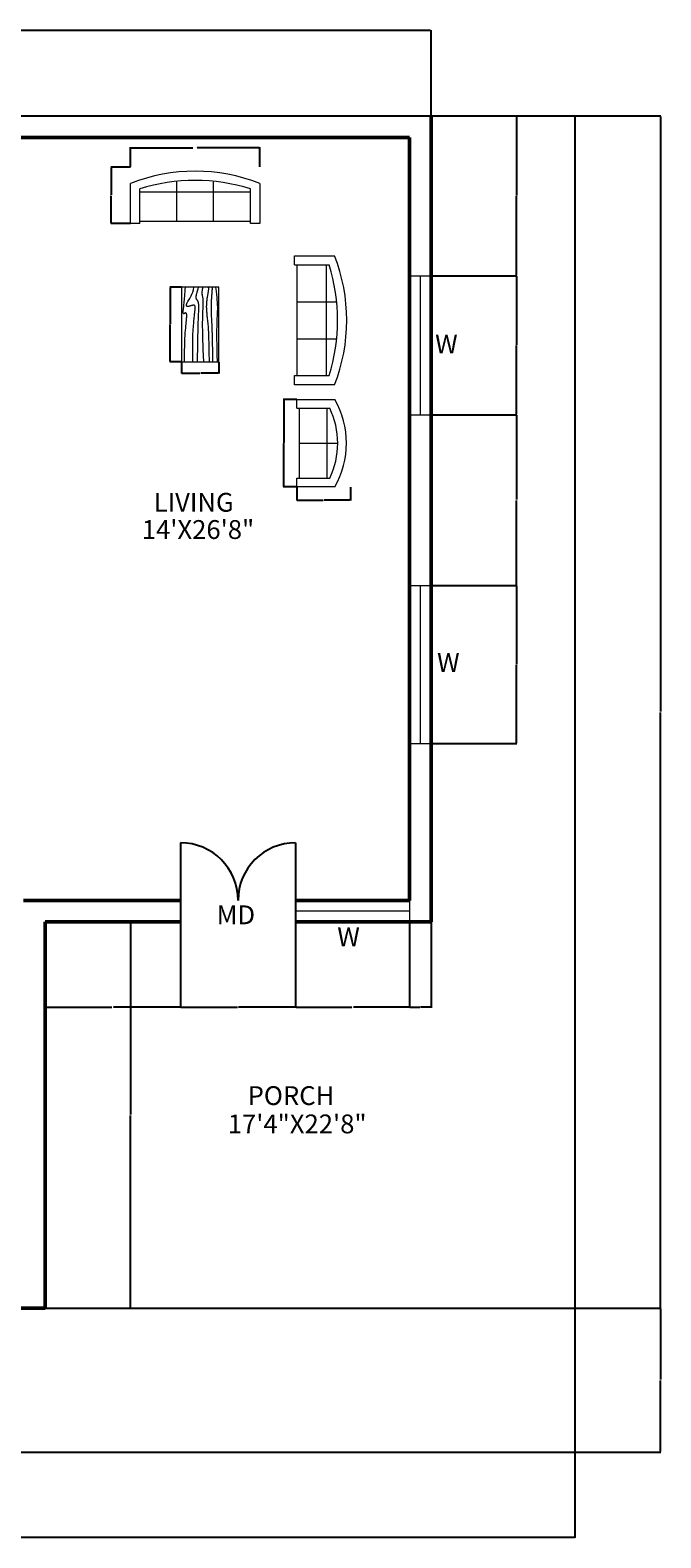
# Model space of a CAD drawing. Units: feet. Extents: x 1544 to 2324, y 1847 to 2475.
# Tile 4 of 4: x 2061 to 2324, y 1847 to 2475. Entities that reach past the tile are written whole.
import ezdxf

# ---------------------------------------------------------------- set-up
doc = ezdxf.new("R2010")
doc.units = ezdxf.units.FT
for name, color, linetype, lineweight in [('A-ANNO-DIMS', 2, 'Continuous', 18), ('A-ANNO-TEXT', 7, 'Continuous', 18), ('A-AREA-IDEN', 7, 'Continuous', 20), ('A-DOOR', 4, 'Continuous', 25), ('A-FURN', 8, 'Continuous', 18), ('A-GLAZ', 4, 'Continuous', 18), ('A-WALL', 7, 'Continuous', 50), ('C-PROP', 3, 'Continuous', 25)]:
    doc.layers.add(name, color=color, linetype=linetype, lineweight=lineweight)
doc.styles.get("Standard").update_dxf_attribs({"font": 'arial.ttf'})
doc.dimstyles.get("Standard").update_dxf_attribs({"dimtxt": 0.18, "dimasz": 0.18, "dimexe": 0.18, "dimexo": 0.0625, "dimgap": 0.09, "dimtad": 0, "dimtih": 1, "dimtoh": 1, "dimdec": 4, "dimzin": 0, "dimdsep": 46, "dimtxsty": 'Standard', "dimcen": 0.09, "dimadec": 0, "dimazin": 0, "dimtfac": 1, "dimtdec": 4, "dimtofl": 0, "dimtmove": 0, "dimatfit": 3, "dimfxl": 1, "dimtolj": 1, "dimtzin": 0, "dimarcsym": 0})

# ---------------------------------------------------------------- blocks, each defined once
blk = doc.blocks.new('Sofa - Roundback 7 ft.')
for p, q in [((-12.00002, -32.4421), (-12.00003, -6.5971)), ((11.99997, -32.4421), (11.99998, -6.5971)), ((-36.000027, -34), (-36.000027, -11.4696)), ((-35.999844, -13.3819), (35.9998, -13.3819)), ((35.99998, -34), (35.99998, -11.4696)), ((-36.000027, -32.4421), (35.99998, -32.4421))]:
    blk.add_line(p, q)
for points in [[(-36.000027, -34), (-42.000027, -34), (-42.000027, -8)], [(41.99998, -8), (41.99998, -34), (35.99998, -34)]]:
    blk.add_lwpolyline(points)
for centre, radius, start, end in [((0, -114.25), 114.25, 68.43141, 111.5686), ((-0.00001, -127.1968), 121.1968, 72.72033, 107.2797)]:
    blk.add_arc(centre, radius, start, end)
blk = doc.blocks.new('Sofa - Roundback Loveseat 5 ft.')
for p, q in [((0, -32.44198), (0, -5.99998)), ((-24, -33.99998), (-24, -11.46958)), ((-23.9998, -13.38178), (23.99986, -13.38178)), ((24.00004, -33.99998), (24.00004, -11.46958)), ((-24, -32.44198), (24.00004, -32.44198))]:
    blk.add_line(p, q)
for points in [[(-24, -33.99998), (-30, -33.99998), (-30, -7.99998)], [(30.00004, -7.99998), (30.00004, -33.99998), (24.00004, -33.99998)]]:
    blk.add_lwpolyline(points)
for centre, radius, start, end in [((0, -60.24998), 60.24998, 60.13715, 119.8628), ((0, -61.38438), 55.38444, 64.32083, 115.6792)]:
    blk.add_arc(centre, radius, start, end)
blk = doc.blocks.new('Table - Rectangular Woodgrain 60 x 30 in.')
for p, q in [((0, 0), (0, -30)), ((60, 0), (0, 0)), ((60, -30), (60, 0)), ((0, -30), (60, -30))]:
    blk.add_line(p, q)
for points in [[(0, -2.4), (4.8155, -2.418), (9.0302, -2.4688), (12.709, -2.5477), (15.9167, -2.65), (18.7181, -2.7711), (21.1781, -2.9063), (23.3616, -3.0508), (25.3333, -3.2), (27.1477, -3.3495), (28.8172, -3.4958), (30.3437, -3.636), (31.7291, -3.7667), (32.9756, -3.8849), (34.0849, -3.9875), (35.059, -4.0714), (35.9, -4.1334), (36.6114, -4.1711), (37.2041, -4.1854), (37.6906, -4.1779), (38.0833, -4.15), (38.3948, -4.1034), (38.6375, -4.0396), (38.8239, -3.9602), (38.9666, -3.8667), (39.0764, -3.7608), (39.1573, -3.6448), (39.2116, -3.521), (39.2416, -3.3917), (39.2498, -3.2593), (39.2385, -3.1261), (39.21, -2.9944), (39.1666, -2.8667), (39.111, -2.7447), (39.0468, -2.6281), (38.978, -2.5163), (38.9083, -2.4083), (38.8418, -2.3035), (38.7823, -2.201), (38.7337, -2.1001), (38.7, -2), (38.6844, -1.9003), (38.6875, -1.8021), (38.7094, -1.707), (38.75, -1.6167), (38.8094, -1.5326), (38.8875, -1.4563), (38.9844, -1.3893), (39.1, -1.3333), (39.2351, -1.2896), (39.3937, -1.2583), (39.5804, -1.2396), (39.8, -1.2333), (40.057, -1.2396), (40.3562, -1.2583), (40.7023, -1.2896), (41.1, -1.3333), (41.5547, -1.3895), (42.0755, -1.4573), (42.6721, -1.5361), (43.3542, -1.625), (44.1316, -1.7233), (45.014, -1.8302), (46.0114, -1.9449), (47.1333, -2.0667), (48.3862, -2.1947), (49.7625, -2.3281), (51.2513, -2.4663), (52.8416, -2.6083), (54.5226, -2.7535), (56.2833, -2.9011), (58.1127, -3.0501), (60, -3.2)], [(0, -9.2), (6.5759, -9.0858), (11.9385, -9.0365), (16.2527, -9.0418), (19.6833, -9.0917), (22.3952, -9.1759), (24.5531, -9.2844), (26.322, -9.4069), (27.8666, -9.5333), (29.3241, -9.6553), (30.7203, -9.7719), (32.0532, -9.8837), (33.3208, -9.9917), (34.5213, -10.0965), (35.6526, -10.199), (36.7128, -10.2999), (37.7, -10.4), (38.6129, -10.4996), (39.4531, -10.5969), (40.223, -10.6895), (40.925, -10.775), (41.5613, -10.8512), (42.1344, -10.9156), (42.6465, -10.966), (43.1, -11), (43.4976, -11.0158), (43.8437, -11.0136), (44.143, -10.9942), (44.4, -10.9583), (44.6195, -10.9069), (44.8062, -10.8406), (44.9648, -10.7603), (45.1, -10.6667), (45.2155, -10.5598), (45.3114, -10.4365), (45.3871, -10.2929), (45.4416, -10.125), (45.4743, -9.929), (45.4844, -9.7011), (45.4709, -9.4371), (45.4333, -9.1333), (45.3716, -8.7883), (45.2896, -8.4104), (45.1919, -8.0107), (45.0833, -7.6), (44.9685, -7.1893), (44.8521, -6.7896), (44.7388, -6.4117), (44.6333, -6.0667), (44.54, -5.7628), (44.4614, -5.4979), (44.4001, -5.2675), (44.3583, -5.0667), (44.3384, -4.8909), (44.3427, -4.7354), (44.3736, -4.5956), (44.4333, -4.4667), (44.5236, -4.3453), (44.6427, -4.2333), (44.7884, -4.1339), (44.9583, -4.05), (45.1501, -3.9849), (45.3614, -3.9417), (45.59, -3.9234), (45.8333, -3.9333), (46.0915, -3.9749), (46.3734, -4.0531), (46.6906, -4.1736), (47.0542, -4.3417), (47.4756, -4.5629), (47.9661, -4.8427), (48.5372, -5.1866), (49.2, -5.6), (49.9676, -6.0844), (50.8594, -6.625), (51.8965, -7.2031), (53.1, -7.8), (54.491, -8.3969), (56.0906, -8.975), (57.9199, -9.5156), (60, -10)], [(0, -12.8), (5.1847, -12.9322), (9.6213, -13.0323), (13.3963, -13.1059), (16.5958, -13.1583), (19.3063, -13.1952), (21.614, -13.2219), (23.6054, -13.2439), (25.3666, -13.2667), (26.9728, -13.2947), (28.4531, -13.3281), (29.8256, -13.3663), (31.1083, -13.4083), (32.3191, -13.4535), (33.476, -13.501), (34.597, -13.5501), (35.7, -13.6), (36.7984, -13.6497), (37.8875, -13.6979), (38.9578, -13.743), (40, -13.7833), (41.0047, -13.8174), (41.9625, -13.8438), (42.864, -13.8607), (43.7, -13.8667), (44.4631, -13.8604), (45.1552, -13.8417), (45.7801, -13.8104), (46.3416, -13.7667), (46.8439, -13.7104), (47.2906, -13.6417), (47.6858, -13.5604), (48.0333, -13.4667), (48.3375, -13.3608), (48.6042, -13.2448), (48.8396, -13.121), (49.05, -12.9917), (49.2417, -12.8593), (49.4208, -12.7261), (49.5937, -12.5944), (49.7667, -12.4667), (49.9452, -12.3451), (50.1323, -12.2313), (50.3303, -12.1268), (50.5416, -12.0333), (50.7686, -11.9524), (51.0135, -11.8854), (51.2788, -11.8341), (51.5666, -11.8), (51.8785, -11.7843), (52.2116, -11.7865), (52.562, -11.8059), (52.926, -11.8417), (53.2998, -11.8931), (53.6795, -11.9594), (54.0614, -12.0397), (54.4416, -12.1333), (54.8223, -12.2401), (55.2293, -12.3625), (55.6942, -12.5037), (56.2489, -12.6667), (56.9251, -12.8547), (57.7545, -13.0708), (58.7689, -13.3182), (60, -13.6)], [(0, -18), (5.124, -17.7273), (9.6609, -17.5057), (13.6705, -17.3303), (17.2125, -17.1958), (20.3467, -17.0973), (23.1328, -17.0297), (25.6307, -16.9878), (27.9, -16.9667), (29.9928, -16.9617), (31.9302, -16.9703), (33.7254, -16.9907), (35.3917, -17.0208), (36.9423, -17.0588), (38.3906, -17.1026), (39.7499, -17.1503), (41.0333, -17.2), (42.2519, -17.2496), (43.4073, -17.2969), (44.4986, -17.3395), (45.525, -17.375), (46.4858, -17.4012), (47.3802, -17.4156), (48.2074, -17.416), (48.9667, -17.4), (49.6583, -17.3662), (50.2872, -17.3167), (50.8595, -17.2547), (51.3812, -17.1833), (51.8584, -17.1057), (52.2971, -17.025), (52.7034, -16.9443), (53.0833, -16.8667), (53.443, -16.7951), (53.789, -16.7313), (54.128, -16.6768), (54.4666, -16.6334), (54.8115, -16.6024), (55.1693, -16.5854), (55.5465, -16.5841), (55.95, -16.6), (56.3828, -16.6337), (56.8346, -16.6823), (57.2915, -16.7418), (57.7396, -16.8084), (58.165, -16.878), (58.5539, -16.9469), (58.8924, -17.0111), (59.1666, -17.0667), (59.3679, -17.1107), (59.5078, -17.1438), (59.6032, -17.1675), (59.6708, -17.1833), (59.7275, -17.193), (59.7901, -17.1979), (59.8753, -17.1998), (60, -17.2)], [(0, -22.4), (8.0098, -22.2501), (14.4094, -22.1011), (19.4168, -21.9535), (23.25, -21.8083), (26.1269, -21.6663), (28.2656, -21.5281), (29.884, -21.3947), (31.2, -21.2667), (32.3967, -21.1448), (33.5172, -21.0292), (34.5697, -20.9198), (35.5625, -20.8167), (36.5037, -20.7198), (37.4015, -20.6292), (38.2642, -20.5448), (39.1, -20.4667), (39.9164, -20.3951), (40.7187, -20.3313), (41.5117, -20.2768), (42.3, -20.2333), (43.0883, -20.2024), (43.8812, -20.1854), (44.6836, -20.1841), (45.5, -20.2), (46.3328, -20.234), (47.1747, -20.2844), (48.0163, -20.3488), (48.8479, -20.425), (49.66, -20.5106), (50.4429, -20.6031), (51.1872, -20.7004), (51.8833, -20.8), (52.5246, -20.8999), (53.1166, -20.9995), (53.6681, -21.0983), (54.1875, -21.1958), (54.6834, -21.2919), (55.1646, -21.3859), (55.6394, -21.4777), (56.1167, -21.5667), (56.6028, -21.6515), (57.0961, -21.7266), (57.5929, -21.7852), (58.0896, -21.8208), (58.5823, -21.8268), (59.0674, -21.7964), (59.5412, -21.723), (60, -21.6)], [(0, -25.2), (8.6355, -25.0504), (15.7026, -24.9031), (21.4049, -24.7606), (25.9458, -24.625), (29.529, -24.4988), (32.3578, -24.3844), (34.6359, -24.284), (36.5667, -24.2), (38.3213, -24.1341), (39.9417, -24.0854), (41.437, -24.0523), (42.8167, -24.0333), (44.0901, -24.0268), (45.2667, -24.0313), (46.3557, -24.0451), (47.3667, -24.0667), (48.309, -24.0947), (49.1928, -24.1287), (50.0284, -24.168), (50.826, -24.2125), (51.5959, -24.2617), (52.3483, -24.3151), (53.0935, -24.3725), (53.8417, -24.4334), (54.6009, -24.497), (55.3699, -24.561), (56.1454, -24.6226), (56.9239, -24.6792), (57.7021, -24.7279), (58.4764, -24.7662), (59.2435, -24.7911), (60, -24.8)], [(0, -28.8), (5.6867, -28.6681), (10.45, -28.5698), (14.407, -28.5012), (17.675, -28.4584), (20.3711, -28.4374), (22.6125, -28.4344), (24.5164, -28.4455), (26.2, -28.4667), (27.762, -28.4947), (29.2276, -28.5281), (30.6033, -28.5663), (31.8958, -28.6084), (33.1118, -28.6535), (34.2578, -28.7011), (35.3405, -28.7501), (36.3666, -28.8), (37.3443, -28.8497), (38.288, -28.8974), (39.2137, -28.9412), (40.1375, -28.9792), (41.0753, -29.0093), (42.0432, -29.0297), (43.0572, -29.0384), (44.1333, -29.0333), (45.2936, -29.0114), (46.5843, -28.9641), (48.0579, -28.8816), (49.7666, -28.7542), (51.7629, -28.5721), (54.0989, -28.3255), (56.8272, -28.0048), (60, -27.6)]]:
    blk.add_lwpolyline(points)
blk = doc.blocks.new('*D19')
at = {"layer": 'A-ANNO-DIMS', "color": 0, "lineweight": -2, "transparency": 16777216}
for p, q in [((2103.25, 2418.42), (2103.25, 2426.61)), ((2103.43, 2426.43), (2129.26, 2426.43)), ((2156.89, 2426.43), (2131.06, 2426.43)), ((2157.07, 2418.42), (2157.07, 2426.61))]:
    blk.add_line(p, q, dxfattribs=at)
at = {"layer": 'A-ANNO-DIMS', "color": 0, "transparency": 16777216}
for points in [[(2103.43, 2426.46), (2103.43, 2426.4), (2103.25, 2426.43)], [(2156.89, 2426.46), (2156.89, 2426.4), (2157.07, 2426.43)]]:
    blk.add_solid(points, dxfattribs=at)
at = {"layer": 'Defpoints', "color": 0, "transparency": 16777216}
for p in [(2157.07, 2426.43), (2103.25, 2418.36), (2157.07, 2418.36)]:
    blk.add_point(p, dxfattribs=at)
at = {"layer": 'A-ANNO-DIMS', "color": 0, "transparency": 16777216, "insert": (2130.16, 2426.43), "char_height": 0.18, "attachment_point": 5}
blk.add_mtext('\\A1;SOFA 54 TYP.', dxfattribs=at)
blk = doc.blocks.new('*D20')
at = {"layer": 'A-ANNO-DIMS', "color": 0, "lineweight": -2, "transparency": 16777216}
for p, q in [((2103.19, 2418.36), (2094.99, 2418.36)), ((2095.17, 2418.18), (2095.17, 2406.79)), ((2095.17, 2395.04), (2095.17, 2406.43)), ((2103.19, 2394.86), (2094.99, 2394.86))]:
    blk.add_line(p, q, dxfattribs=at)
at = {"layer": 'A-ANNO-DIMS', "color": 0, "transparency": 16777216}
for points in [[(2095.14, 2418.18), (2095.2, 2418.18), (2095.17, 2418.36)], [(2095.14, 2395.04), (2095.2, 2395.04), (2095.17, 2394.86)]]:
    blk.add_solid(points, dxfattribs=at)
at = {"layer": 'Defpoints', "color": 0, "transparency": 16777216}
for p in [(2095.17, 2418.36), (2103.25, 2418.36), (2103.25, 2394.86)]:
    blk.add_point(p, dxfattribs=at)
at = {"layer": 'A-ANNO-DIMS', "color": 0, "transparency": 16777216, "insert": (2095.17, 2406.61), "char_height": 0.18, "attachment_point": 5}
blk.add_mtext('\\A1;23 TYP.', dxfattribs=at)
blk = doc.blocks.new('*D25')
at = {"layer": 'A-ANNO-DIMS', "color": 0, "lineweight": -2, "transparency": 16777216}
for p, q in [((2172.52, 2321.52), (2166.92, 2321.52)), ((2167.1, 2321.34), (2167.1, 2303.44)), ((2167.1, 2285.18), (2167.1, 2303.07)), ((2172.52, 2285), (2166.92, 2285))]:
    blk.add_line(p, q, dxfattribs=at)
at = {"layer": 'A-ANNO-DIMS', "color": 0, "transparency": 16777216}
for points in [[(2167.07, 2321.34), (2167.13, 2321.34), (2167.1, 2321.52)], [(2167.07, 2285.18), (2167.13, 2285.18), (2167.1, 2285)]]:
    blk.add_solid(points, dxfattribs=at)
at = {"layer": 'Defpoints', "color": 0, "transparency": 16777216}
for p in [(2172.58, 2321.52), (2167.1, 2285), (2172.58, 2285)]:
    blk.add_point(p, dxfattribs=at)
at = {"layer": 'A-ANNO-DIMS', "color": 0, "transparency": 16777216, "insert": (2167.1, 2303.26), "char_height": 0.18, "attachment_point": 5}
blk.add_mtext('\\A1;LOVESEAT 37', dxfattribs=at)
blk = doc.blocks.new('*D26')
at = {"layer": 'A-ANNO-DIMS', "color": 0, "lineweight": -2, "transparency": 16777216}
for p, q in [((2172.58, 2284.94), (2172.58, 2279.34)), ((2194.89, 2284.94), (2194.89, 2279.34)), ((2172.76, 2279.52), (2183.52, 2279.52)), ((2194.71, 2279.52), (2183.96, 2279.52))]:
    blk.add_line(p, q, dxfattribs=at)
at = {"layer": 'A-ANNO-DIMS', "color": 0, "transparency": 16777216}
for points in [[(2172.76, 2279.55), (2172.76, 2279.49), (2172.58, 2279.52)], [(2194.71, 2279.55), (2194.71, 2279.49), (2194.89, 2279.52)]]:
    blk.add_solid(points, dxfattribs=at)
at = {"layer": 'Defpoints', "color": 0, "transparency": 16777216}
for p in [(2172.58, 2285), (2194.89, 2285), (2194.89, 2279.52)]:
    blk.add_point(p, dxfattribs=at)
at = {"layer": 'A-ANNO-DIMS', "color": 0, "transparency": 16777216, "insert": (2183.74, 2279.52), "char_height": 0.18, "attachment_point": 5}
blk.add_mtext('\\A1;22', dxfattribs=at)
blk = doc.blocks.new('*D27')
at = {"layer": 'A-ANNO-DIMS', "color": 0, "lineweight": -2, "transparency": 16777216}
for p, q in [((2124.42, 2368.31), (2119.63, 2368.31)), ((2119.81, 2368.13), (2119.81, 2352.92)), ((2119.81, 2337.34), (2119.81, 2352.55)), ((2124.42, 2337.16), (2119.63, 2337.16))]:
    blk.add_line(p, q, dxfattribs=at)
at = {"layer": 'A-ANNO-DIMS', "color": 0, "transparency": 16777216}
for points in [[(2119.78, 2368.13), (2119.84, 2368.13), (2119.81, 2368.31)], [(2119.78, 2337.34), (2119.84, 2337.34), (2119.81, 2337.16)]]:
    blk.add_solid(points, dxfattribs=at)
at = {"layer": 'Defpoints', "color": 0, "transparency": 16777216}
for p in [(2119.81, 2368.31), (2124.48, 2368.31), (2124.48, 2337.16)]:
    blk.add_point(p, dxfattribs=at)
at = {"layer": 'A-ANNO-DIMS', "color": 0, "transparency": 16777216, "insert": (2119.81, 2352.73), "char_height": 0.18, "attachment_point": 5}
blk.add_mtext('\\A1;TABLE 31', dxfattribs=at)
blk = doc.blocks.new('*D28')
at = {"layer": 'A-ANNO-DIMS', "color": 0, "lineweight": -2, "transparency": 16777216}
for p, q in [((2124.48, 2337.1), (2124.48, 2332.31)), ((2124.66, 2332.49), (2132.06, 2332.49)), ((2139.88, 2332.49), (2132.48, 2332.49)), ((2140.06, 2337.1), (2140.06, 2332.31))]:
    blk.add_line(p, q, dxfattribs=at)
at = {"layer": 'A-ANNO-DIMS', "color": 0, "transparency": 16777216}
for points in [[(2124.66, 2332.52), (2124.66, 2332.46), (2124.48, 2332.49)], [(2139.88, 2332.52), (2139.88, 2332.46), (2140.06, 2332.49)]]:
    blk.add_solid(points, dxfattribs=at)
at = {"layer": 'Defpoints', "color": 0, "transparency": 16777216}
for p in [(2124.48, 2337.16), (2124.48, 2332.49), (2140.06, 2337.16)]:
    blk.add_point(p, dxfattribs=at)
at = {"layer": 'A-ANNO-DIMS', "color": 0, "transparency": 16777216, "insert": (2132.27, 2332.49), "char_height": 0.18, "attachment_point": 5}
blk.add_mtext('\\A1;16', dxfattribs=at)
blk = doc.blocks.new('*D31')
at = {"layer": 'A-ANNO-DIMS', "color": 0, "lineweight": -2, "transparency": 16777216}
for p, q in [((1579.55, 1882.61), (1579.55, 1846.89)), ((2288.55, 1882.61), (2288.55, 1846.89)), ((1579.73, 1847.07), (1933.77, 1847.07)), ((2288.37, 1847.07), (1934.34, 1847.07))]:
    blk.add_line(p, q, dxfattribs=at)
at = {"layer": 'A-ANNO-DIMS', "color": 0, "transparency": 16777216}
for points in [[(1579.73, 1847.1), (1579.73, 1847.04), (1579.55, 1847.07)], [(2288.37, 1847.1), (2288.37, 1847.04), (2288.55, 1847.07)]]:
    blk.add_solid(points, dxfattribs=at)
at = {"layer": 'Defpoints', "color": 0, "transparency": 16777216}
for p in [(1579.55, 1882.67), (2288.55, 1882.67), (2288.55, 1847.07)]:
    blk.add_point(p, dxfattribs=at)
at = {"layer": 'A-ANNO-DIMS', "color": 0, "transparency": 16777216, "insert": (1934.05, 1847.07), "char_height": 0.18, "attachment_point": 5}
blk.add_mtext('\\A1;709', dxfattribs=at)
blk = doc.blocks.new('*D33')
at = {"layer": 'A-ANNO-DIMS', "color": 0, "lineweight": -2, "transparency": 16777216}
for p, q in [((1639.55, 2387.73), (1639.55, 2475.45)), ((1639.73, 2475.27), (1933.76, 2475.27)), ((2228.37, 2475.27), (1934.34, 2475.27)), ((2228.55, 2439.73), (2228.55, 2475.45))]:
    blk.add_line(p, q, dxfattribs=at)
at = {"layer": 'A-ANNO-DIMS', "color": 0, "transparency": 16777216}
for points in [[(1639.73, 2475.3), (1639.73, 2475.24), (1639.55, 2475.27)], [(2228.37, 2475.3), (2228.37, 2475.24), (2228.55, 2475.27)]]:
    blk.add_solid(points, dxfattribs=at)
at = {"layer": 'Defpoints', "color": 0, "transparency": 16777216}
for p in [(2228.55, 2475.27), (2228.55, 2439.67), (1639.55, 2387.67)]:
    blk.add_point(p, dxfattribs=at)
at = {"layer": 'A-ANNO-DIMS', "color": 0, "transparency": 16777216, "insert": (1934.05, 2475.27), "char_height": 0.18, "attachment_point": 5}
blk.add_mtext('\\A1;589', dxfattribs=at)
blk = doc.blocks.new('*D34')
at = {"layer": 'A-ANNO-DIMS', "color": 0, "lineweight": -2, "transparency": 16777216}
for p, q in [((2228.62, 2439.67), (2324.33, 2439.67)), ((2324.15, 2439.49), (2324.15, 2191.35)), ((2324.15, 1942.85), (2324.15, 2190.99)), ((2067.62, 1942.67), (2324.33, 1942.67))]:
    blk.add_line(p, q, dxfattribs=at)
at = {"layer": 'A-ANNO-DIMS', "color": 0, "transparency": 16777216}
for points in [[(2324.12, 2439.49), (2324.18, 2439.49), (2324.15, 2439.67)], [(2324.12, 1942.85), (2324.18, 1942.85), (2324.15, 1942.67)]]:
    blk.add_solid(points, dxfattribs=at)
at = {"layer": 'Defpoints', "color": 0, "transparency": 16777216}
for p in [(2228.55, 2439.67), (2324.15, 2439.67), (2067.55, 1942.67)]:
    blk.add_point(p, dxfattribs=at)
at = {"layer": 'A-ANNO-DIMS', "color": 0, "transparency": 16777216, "insert": (2324.15, 2191.17), "char_height": 0.18, "attachment_point": 5}
blk.add_mtext('\\A1;497', dxfattribs=at)
blk = doc.blocks.new('*D36')
at = {"layer": 'A-ANNO-DIMS', "color": 0, "lineweight": -2, "transparency": 16777216}
for p, q in [((2067.62, 1942.67), (2324.33, 1942.67)), ((2324.15, 1942.49), (2324.15, 1912.85)), ((2324.15, 1882.85), (2324.15, 1912.49)), ((2288.62, 1882.67), (2324.33, 1882.67))]:
    blk.add_line(p, q, dxfattribs=at)
at = {"layer": 'A-ANNO-DIMS', "color": 0, "transparency": 16777216}
for points in [[(2324.12, 1942.49), (2324.18, 1942.49), (2324.15, 1942.67)], [(2324.12, 1882.85), (2324.18, 1882.85), (2324.15, 1882.67)]]:
    blk.add_solid(points, dxfattribs=at)
at = {"layer": 'Defpoints', "color": 0, "transparency": 16777216}
for p in [(2067.55, 1942.67), (2288.55, 1882.67), (2324.15, 1882.67)]:
    blk.add_point(p, dxfattribs=at)
at = {"layer": 'A-ANNO-DIMS', "color": 0, "transparency": 16777216, "insert": (2324.15, 1912.67), "char_height": 0.18, "attachment_point": 5}
blk.add_mtext('\\A1;60', dxfattribs=at)
blk = doc.blocks.new('*D44')
at = {"layer": 'A-ANNO-DIMS', "color": 0, "lineweight": -2, "transparency": 16777216}
for p, q in [((2228.62, 2439.67), (2264.33, 2439.67)), ((2264.15, 2439.49), (2264.15, 2406.55)), ((2264.15, 2373.25), (2264.15, 2406.19)), ((2228.62, 2373.07), (2264.33, 2373.07))]:
    blk.add_line(p, q, dxfattribs=at)
at = {"layer": 'A-ANNO-DIMS', "color": 0, "transparency": 16777216}
for points in [[(2264.12, 2439.49), (2264.18, 2439.49), (2264.15, 2439.67)], [(2264.12, 2373.25), (2264.18, 2373.25), (2264.15, 2373.07)]]:
    blk.add_solid(points, dxfattribs=at)
at = {"layer": 'Defpoints', "color": 0, "transparency": 16777216}
for p in [(2228.55, 2439.67), (2228.55, 2373.07), (2264.15, 2373.07)]:
    blk.add_point(p, dxfattribs=at)
at = {"layer": 'A-ANNO-DIMS', "color": 0, "transparency": 16777216, "insert": (2264.15, 2406.37), "char_height": 0.18, "attachment_point": 5}
blk.add_mtext('\\A1;66.6', dxfattribs=at)
blk = doc.blocks.new('*D45')
at = {"layer": 'A-ANNO-DIMS', "color": 0, "lineweight": -2, "transparency": 16777216}
for p, q in [((2228.62, 2373.07), (2264.33, 2373.07)), ((2264.15, 2372.89), (2264.15, 2344.29)), ((2264.15, 2315.32), (2264.15, 2343.92)), ((2228.62, 2315.14), (2264.33, 2315.14))]:
    blk.add_line(p, q, dxfattribs=at)
at = {"layer": 'A-ANNO-DIMS', "color": 0, "transparency": 16777216}
for points in [[(2264.12, 2372.89), (2264.18, 2372.89), (2264.15, 2373.07)], [(2264.12, 2315.32), (2264.18, 2315.32), (2264.15, 2315.14)]]:
    blk.add_solid(points, dxfattribs=at)
at = {"layer": 'Defpoints', "color": 0, "transparency": 16777216}
for p in [(2228.55, 2373.07), (2228.55, 2315.14), (2264.15, 2315.14)]:
    blk.add_point(p, dxfattribs=at)
at = {"layer": 'A-ANNO-DIMS', "color": 0, "transparency": 16777216, "insert": (2264.15, 2344.1), "char_height": 0.18, "attachment_point": 5}
blk.add_mtext('\\A1;57.94', dxfattribs=at)
blk = doc.blocks.new('*D46')
at = {"layer": 'A-ANNO-DIMS', "color": 0, "lineweight": -2, "transparency": 16777216}
for p, q in [((2228.62, 2315.14), (2264.33, 2315.14)), ((2264.15, 2314.96), (2264.15, 2279.71)), ((2264.15, 2244.1), (2264.15, 2279.35)), ((2228.62, 2243.92), (2264.33, 2243.92))]:
    blk.add_line(p, q, dxfattribs=at)
at = {"layer": 'A-ANNO-DIMS', "color": 0, "transparency": 16777216}
for points in [[(2264.12, 2314.96), (2264.18, 2314.96), (2264.15, 2315.14)], [(2264.12, 2244.1), (2264.18, 2244.1), (2264.15, 2243.92)]]:
    blk.add_solid(points, dxfattribs=at)
at = {"layer": 'Defpoints', "color": 0, "transparency": 16777216}
for p in [(2228.55, 2315.14), (2228.55, 2243.92), (2264.15, 2243.92)]:
    blk.add_point(p, dxfattribs=at)
at = {"layer": 'A-ANNO-DIMS', "color": 0, "transparency": 16777216, "insert": (2264.15, 2279.53), "char_height": 0.18, "attachment_point": 5}
blk.add_mtext('\\A1;71.21', dxfattribs=at)
blk = doc.blocks.new('*D47')
at = {"layer": 'A-ANNO-DIMS', "color": 0, "lineweight": -2, "transparency": 16777216}
for p, q in [((2228.62, 2243.92), (2264.33, 2243.92)), ((2264.15, 2243.74), (2264.15, 2211.15)), ((2264.15, 2178.2), (2264.15, 2210.79)), ((2228.62, 2178.02), (2264.33, 2178.02))]:
    blk.add_line(p, q, dxfattribs=at)
at = {"layer": 'A-ANNO-DIMS', "color": 0, "transparency": 16777216}
for points in [[(2264.12, 2243.74), (2264.18, 2243.74), (2264.15, 2243.92)], [(2264.12, 2178.2), (2264.18, 2178.2), (2264.15, 2178.02)]]:
    blk.add_solid(points, dxfattribs=at)
at = {"layer": 'Defpoints', "color": 0, "transparency": 16777216}
for p in [(2228.55, 2243.92), (2228.55, 2178.02), (2264.15, 2178.02)]:
    blk.add_point(p, dxfattribs=at)
at = {"layer": 'A-ANNO-DIMS', "color": 0, "transparency": 16777216, "insert": (2264.15, 2210.97), "char_height": 0.18, "attachment_point": 5}
blk.add_mtext('\\A1;65.9', dxfattribs=at)
blk = doc.blocks.new('*D48')
at = {"layer": 'A-ANNO-DIMS', "color": 0, "lineweight": -2, "transparency": 16777216}
for p, q in [((2067.62, 2103.67), (2103.33, 2103.67)), ((2103.15, 2103.49), (2103.15, 2023.35)), ((2103.15, 1942.85), (2103.15, 2022.99)), ((2067.62, 1942.67), (2103.33, 1942.67))]:
    blk.add_line(p, q, dxfattribs=at)
at = {"layer": 'A-ANNO-DIMS', "color": 0, "transparency": 16777216}
for points in [[(2103.12, 2103.49), (2103.18, 2103.49), (2103.15, 2103.67)], [(2103.12, 1942.85), (2103.18, 1942.85), (2103.15, 1942.67)]]:
    blk.add_solid(points, dxfattribs=at)
at = {"layer": 'Defpoints', "color": 0, "transparency": 16777216}
for p in [(2067.55, 2103.67), (2067.55, 1942.67), (2103.15, 1942.67)]:
    blk.add_point(p, dxfattribs=at)
at = {"layer": 'A-ANNO-DIMS', "color": 0, "transparency": 16777216, "insert": (2103.15, 2023.17), "char_height": 0.18, "attachment_point": 5}
blk.add_mtext('\\A1;161', dxfattribs=at)
blk = doc.blocks.new('*D49')
at = {"layer": 'A-ANNO-DIMS', "color": 0, "lineweight": -2, "transparency": 16777216}
for p, q in [((2067.55, 2103.61), (2067.55, 2067.89)), ((2124.05, 2103.61), (2124.05, 2067.89)), ((2067.73, 2068.07), (2095.48, 2068.07)), ((2123.87, 2068.07), (2096.13, 2068.07))]:
    blk.add_line(p, q, dxfattribs=at)
at = {"layer": 'A-ANNO-DIMS', "color": 0, "transparency": 16777216}
for points in [[(2067.73, 2068.1), (2067.73, 2068.04), (2067.55, 2068.07)], [(2123.87, 2068.1), (2123.87, 2068.04), (2124.05, 2068.07)]]:
    blk.add_solid(points, dxfattribs=at)
at = {"layer": 'Defpoints', "color": 0, "transparency": 16777216}
for p in [(2067.55, 2103.67), (2124.05, 2103.67), (2067.55, 2068.07)]:
    blk.add_point(p, dxfattribs=at)
at = {"layer": 'A-ANNO-DIMS', "color": 0, "transparency": 16777216, "insert": (2095.8, 2068.07), "char_height": 0.18, "attachment_point": 5}
blk.add_mtext('\\A1;56.5', dxfattribs=at)
blk = doc.blocks.new('*D50')
at = {"layer": 'A-ANNO-DIMS', "color": 0, "lineweight": -2, "transparency": 16777216}
for p, q in [((2124.05, 2103.61), (2124.05, 2067.89)), ((2172.05, 2103.61), (2172.05, 2067.89)), ((2124.23, 2068.07), (2147.83, 2068.07)), ((2171.87, 2068.07), (2148.28, 2068.07))]:
    blk.add_line(p, q, dxfattribs=at)
at = {"layer": 'A-ANNO-DIMS', "color": 0, "transparency": 16777216}
for points in [[(2124.23, 2068.1), (2124.23, 2068.04), (2124.05, 2068.07)], [(2171.87, 2068.1), (2171.87, 2068.04), (2172.05, 2068.07)]]:
    blk.add_solid(points, dxfattribs=at)
at = {"layer": 'Defpoints', "color": 0, "transparency": 16777216}
for p in [(2124.05, 2103.67), (2172.05, 2103.67), (2124.05, 2068.07)]:
    blk.add_point(p, dxfattribs=at)
at = {"layer": 'A-ANNO-DIMS', "color": 0, "transparency": 16777216, "insert": (2148.05, 2068.07), "char_height": 0.18, "attachment_point": 5}
blk.add_mtext('\\A1;48', dxfattribs=at)
blk = doc.blocks.new('*D51')
at = {"layer": 'A-ANNO-DIMS', "color": 0, "lineweight": -2, "transparency": 16777216}
for p, q in [((2172.05, 2103.61), (2172.05, 2067.89)), ((2219.55, 2103.61), (2219.55, 2067.89)), ((2172.23, 2068.07), (2195.48, 2068.07)), ((2219.37, 2068.07), (2196.13, 2068.07))]:
    blk.add_line(p, q, dxfattribs=at)
at = {"layer": 'A-ANNO-DIMS', "color": 0, "transparency": 16777216}
for points in [[(2172.23, 2068.1), (2172.23, 2068.04), (2172.05, 2068.07)], [(2219.37, 2068.1), (2219.37, 2068.04), (2219.55, 2068.07)]]:
    blk.add_solid(points, dxfattribs=at)
at = {"layer": 'Defpoints', "color": 0, "transparency": 16777216}
for p in [(2172.05, 2103.67), (2219.55, 2103.67), (2172.05, 2068.07)]:
    blk.add_point(p, dxfattribs=at)
at = {"layer": 'A-ANNO-DIMS', "color": 0, "transparency": 16777216, "insert": (2195.8, 2068.07), "char_height": 0.18, "attachment_point": 5}
blk.add_mtext('\\A1;47.5', dxfattribs=at)
blk = doc.blocks.new('*D52')
at = {"layer": 'A-ANNO-DIMS', "color": 0, "lineweight": -2, "transparency": 16777216}
for p, q in [((2219.55, 2103.61), (2219.55, 2067.89)), ((2228.55, 2103.61), (2228.55, 2067.89)), ((2219.73, 2068.07), (2223.9, 2068.07)), ((2228.37, 2068.07), (2224.2, 2068.07))]:
    blk.add_line(p, q, dxfattribs=at)
at = {"layer": 'A-ANNO-DIMS', "color": 0, "transparency": 16777216}
for points in [[(2219.73, 2068.1), (2219.73, 2068.04), (2219.55, 2068.07)], [(2228.37, 2068.1), (2228.37, 2068.04), (2228.55, 2068.07)]]:
    blk.add_solid(points, dxfattribs=at)
at = {"layer": 'Defpoints', "color": 0, "transparency": 16777216}
for p in [(2219.55, 2103.67), (2228.55, 2103.67), (2219.55, 2068.07)]:
    blk.add_point(p, dxfattribs=at)
at = {"layer": 'A-ANNO-DIMS', "color": 0, "transparency": 16777216, "insert": (2224.05, 2068.07), "char_height": 0.18, "attachment_point": 5}
blk.add_mtext('\\A1;9', dxfattribs=at)

msp = doc.modelspace()

# ---------------------------------------------------------------- linework, layer by layer
at = {"layer": 'A-DOOR'}
for p, q in [((2124.0539, 2136.6692), (2124.0539, 2103.6692)), ((2172.0539, 2136.6692), (2172.0539, 2103.6692))]:
    msp.add_line(p, q, dxfattribs=at)
for centre, start, end in [((2124.0539, 2112.6692), 0, 90), ((2172.0539, 2112.6692), 90, 180)]:
    msp.add_arc(centre, 24, start, end, dxfattribs=at)
at = {"layer": 'A-GLAZ'}
for p, q in [((2219.5539, 2373.0729), (2228.5539, 2373.0729)), ((2224.0539, 2373.0729), (2224.0539, 2315.1354)), ((2219.5539, 2315.1354), (2228.5539, 2315.1354)), ((2219.5539, 2243.9206), (2228.5539, 2243.9206)), ((2224.0539, 2243.9206), (2224.0539, 2178.0199)), ((2219.5539, 2178.0199), (2228.5539, 2178.0199)), ((2219.5539, 2112.6692), (2219.5539, 2103.6692)), ((2219.5539, 2108.1692), (2172.0539, 2108.1692))]:
    msp.add_line(p, q, dxfattribs=at)
at = {"layer": 'A-WALL'}
for p, q in [((2228.5539, 2439.6692), (2228.5539, 2103.6692)), ((2051.5539, 2430.6692), (2219.5539, 2430.6692)), ((2219.5539, 2430.6692), (2219.5539, 2112.6692)), ((2058.5539, 2112.6692), (2124.0539, 2112.6692)), ((2172.0539, 2112.6692), (2219.5539, 2112.6692)), ((2067.5539, 1942.6692), (2067.5539, 2103.6692)), ((2067.5539, 2103.6692), (2124.0539, 2103.6692)), ((2172.0539, 2103.6692), (2228.5539, 2103.6692)), ((2055.5539, 1942.6692), (2067.5539, 1942.6692))]:
    msp.add_line(p, q, dxfattribs=at)
at = {"layer": 'C-PROP'}
for p, q in [((1901.5539, 2439.6692), (2288.5539, 2439.6692)), ((2288.5539, 2439.6692), (2288.5539, 2103.6692)), ((2288.5539, 2103.6692), (2288.5539, 1882.6692)), ((1639.5539, 1882.6692), (2288.5539, 1882.6692))]:
    msp.add_line(p, q, dxfattribs=at)

# ---------------------------------------------------------------- block references
at = {"layer": 'A-FURN', "xscale": 0.6407589581852918, "yscale": 0.6407589581852918, "zscale": 0.6407589581852918}
msp.add_blockref('Sofa - Roundback 7 ft.', (2130.1601, 2416.6498), dxfattribs=at)
at = {"layer": 'A-FURN'}
for name, p, xscale, yscale, zscale, rotation in [('Sofa - Roundback 7 ft.', (2193.382, 2354.4796), 0.6407589581852918, 0.6407589581852918, 0.6407589581852918, 270), ('Table - Rectangular Woodgrain 60 x 30 in.', (2124.4829, 2337.1612), 0.5191134502944525, 0.5191134502944525, 0.5191134502944525, 90), ('Sofa - Roundback Loveseat 5 ft.', (2193.2713, 2303.2578), 0.6086332420955142, 0.6086332420955142, 0.6086332420955142, 270)]:
    msp.add_blockref(name, p, dxfattribs=dict(at, xscale=xscale, yscale=yscale, zscale=zscale, rotation=rotation))

# ---------------------------------------------------------------- texts
at = {"layer": 'A-ANNO-TEXT'}
for s, height, p in [('W', 7.8492, (2230.2271, 2340.6725)), ('W', 7.8492, (2231.0446, 2207.8942)), ('MD', 7.84917, (2139.0975, 2102.7015)), ('W', 7.8492, (2189.4284, 2093.5131))]:
    msp.add_text(s, height=height, dxfattribs=at).set_placement(p)
at = {"layer": 'A-AREA-IDEN'}
for s, height, p in [('LIVING', 7.84917, (2112.8564, 2274.6889)), ('14\'X26\'8"', 7.84917, (2107.9111, 2263.3307)), ('PORCH', 7.84917, (2152.0387, 2027.3255)), ('17\'4"X22\'8"', 7.849169, (2143.7532, 2015.5332))]:
    msp.add_text(s, height=height, dxfattribs=at).set_placement(p)

# ---------------------------------------------------------------- dimensions: what is measured, and where the dimension line sits
at = {"layer": 'A-ANNO-DIMS'}
for base, p1, p2, picture, middle in [((2228.5539, 2475.2692), (1639.5539, 2387.6692), (2228.5539, 2439.6692), '*D33', (1934.0539, 2475.2692)), ((2194.8943, 2279.5211), (2172.5777, 2284.9988), (2194.8943, 2284.9988), '*D26', (2183.736, 2279.5211)), ((2288.5539, 1847.0692), (1579.5539, 1882.6692), (2288.5539, 1882.6692), '*D31', (1934.0539, 1847.0692))]:
    dim = msp.add_linear_dim(base=base, p1=p1, p2=p2, dimstyle='Standard', override={"dimdec": 0, "dimlfac": 1, "dimrnd": 0, "dimzin": 0, "dimdsep": 46, "dimlunit": 2}, dxfattribs=at)
    dim.commit()
    dim.dimension.update_dxf_attribs({"geometry": picture, "text_midpoint": middle})
for base, p1, p2, angle, override, picture, middle in [((2324.1539, 2439.6692), (2067.5539, 1942.6692), (2228.5539, 2439.6692), 90, {"dimdec": 0, "dimlfac": 1, "dimrnd": 0, "dimzin": 0, "dimdsep": 46, "dimlunit": 2}, '*D34', (2324.1539, 2191.1692)), ((2264.1539, 2373.0729), (2228.5539, 2439.6692), (2228.5539, 2373.0729), 270, {"dimdec": 1, "dimlfac": 1, "dimrnd": 0, "dimzin": 0, "dimdsep": 46, "dimlunit": 2}, '*D44', (2264.1539, 2406.371)), ((2264.1539, 2315.1354), (2228.5539, 2373.0729), (2228.5539, 2315.1354), 270, {"dimdec": 2, "dimlfac": 1, "dimrnd": 0, "dimzin": 0, "dimdsep": 46, "dimlunit": 2}, '*D45', (2264.1539, 2344.1041)), ((2124.4829, 2332.4892), (2140.0563, 2337.1612), (2124.4829, 2337.1612), 180, {"dimdec": 0, "dimlfac": 1, "dimrnd": 0, "dimzin": 0, "dimdsep": 46, "dimlunit": 2}, '*D28', (2132.2696, 2332.4892)), ((2264.1539, 2243.9206), (2228.5539, 2315.1354), (2228.5539, 2243.9206), 270, {"dimdec": 2, "dimlfac": 1, "dimrnd": 0, "dimzin": 0, "dimdsep": 46, "dimlunit": 2}, '*D46', (2264.1539, 2279.528)), ((2264.1539, 2178.0199), (2228.5539, 2243.9206), (2228.5539, 2178.0199), 270, {"dimdec": 1, "dimlfac": 1, "dimrnd": 0, "dimzin": 0, "dimdsep": 46, "dimlunit": 2}, '*D47', (2264.1539, 2210.9703)), ((2103.1539, 1942.6692), (2067.5539, 2103.6692), (2067.5539, 1942.6692), 270, {"dimdec": 0, "dimlfac": 1, "dimrnd": 0, "dimzin": 0, "dimdsep": 46, "dimlunit": 2}, '*D48', (2103.1539, 2023.1692)), ((2067.5539, 2068.0692), (2124.0539, 2103.6692), (2067.5539, 2103.6692), 180, {"dimdec": 1, "dimlfac": 1, "dimrnd": 0, "dimzin": 0, "dimdsep": 46, "dimlunit": 2}, '*D49', (2095.8039, 2068.0692)), ((2124.0539, 2068.0692), (2172.0539, 2103.6692), (2124.0539, 2103.6692), 180, {"dimdec": 0, "dimlfac": 1, "dimrnd": 0, "dimzin": 0, "dimdsep": 46, "dimlunit": 2}, '*D50', (2148.0539, 2068.0692)), ((2172.0539, 2068.0692), (2219.5539, 2103.6692), (2172.0539, 2103.6692), 180, {"dimdec": 1, "dimlfac": 1, "dimrnd": 0, "dimzin": 0, "dimdsep": 46, "dimlunit": 2}, '*D51', (2195.8039, 2068.0692)), ((2219.5539, 2068.0692), (2228.5539, 2103.6692), (2219.5539, 2103.6692), 180, {"dimdec": 0, "dimlfac": 1, "dimrnd": 0, "dimzin": 0, "dimdsep": 46, "dimlunit": 2}, '*D52', (2224.0539, 2068.0692)), ((2324.1539, 1882.6692), (2067.5539, 1942.6692), (2288.5539, 1882.6692), 90, {"dimdec": 0, "dimlfac": 1, "dimrnd": 0, "dimzin": 0, "dimdsep": 46, "dimlunit": 2}, '*D36', (2324.1539, 1912.6692))]:
    dim = msp.add_linear_dim(base=base, p1=p1, p2=p2, angle=angle, dimstyle='Standard', override=override, dxfattribs=at)
    dim.commit()
    dim.dimension.update_dxf_attribs({"geometry": picture, "text_midpoint": middle})
dim = msp.add_linear_dim(base=(2157.0719, 2426.432), p1=(2103.2482, 2418.3584), p2=(2157.0719, 2418.3584), text='SOFA <> TYP.', dimstyle='Standard', override={"dimdec": 0, "dimlfac": 1, "dimrnd": 0, "dimzin": 0, "dimdsep": 46, "dimlunit": 2}, dxfattribs=at)
dim.commit()
dim.dimension.update_dxf_attribs({"geometry": '*D19', "text_midpoint": (2130.1601, 2426.432)})
for base, p1, p2, angle, text, picture, middle in [((2095.1746, 2418.3584), (2103.2482, 2394.864), (2103.2482, 2418.3584), 90, '<> TYP.', '*D20', (2095.1746, 2406.6112)), ((2119.8109, 2368.308), (2124.4829, 2337.1612), (2124.4829, 2368.308), 90, 'TABLE <>', '*D27', (2119.8109, 2352.7346)), ((2167.1, 2284.9988), (2172.5777, 2321.5168), (2172.5777, 2284.9988), 270, 'LOVESEAT <>', '*D25', (2167.1, 2303.2578))]:
    dim = msp.add_linear_dim(base=base, p1=p1, p2=p2, angle=angle, text=text, dimstyle='Standard', override={"dimdec": 0, "dimlfac": 1, "dimrnd": 0, "dimzin": 0, "dimdsep": 46, "dimlunit": 2}, dxfattribs=at)
    dim.commit()
    dim.dimension.update_dxf_attribs({"geometry": picture, "text_midpoint": middle})

doc.saveas('drawing.dxf')
